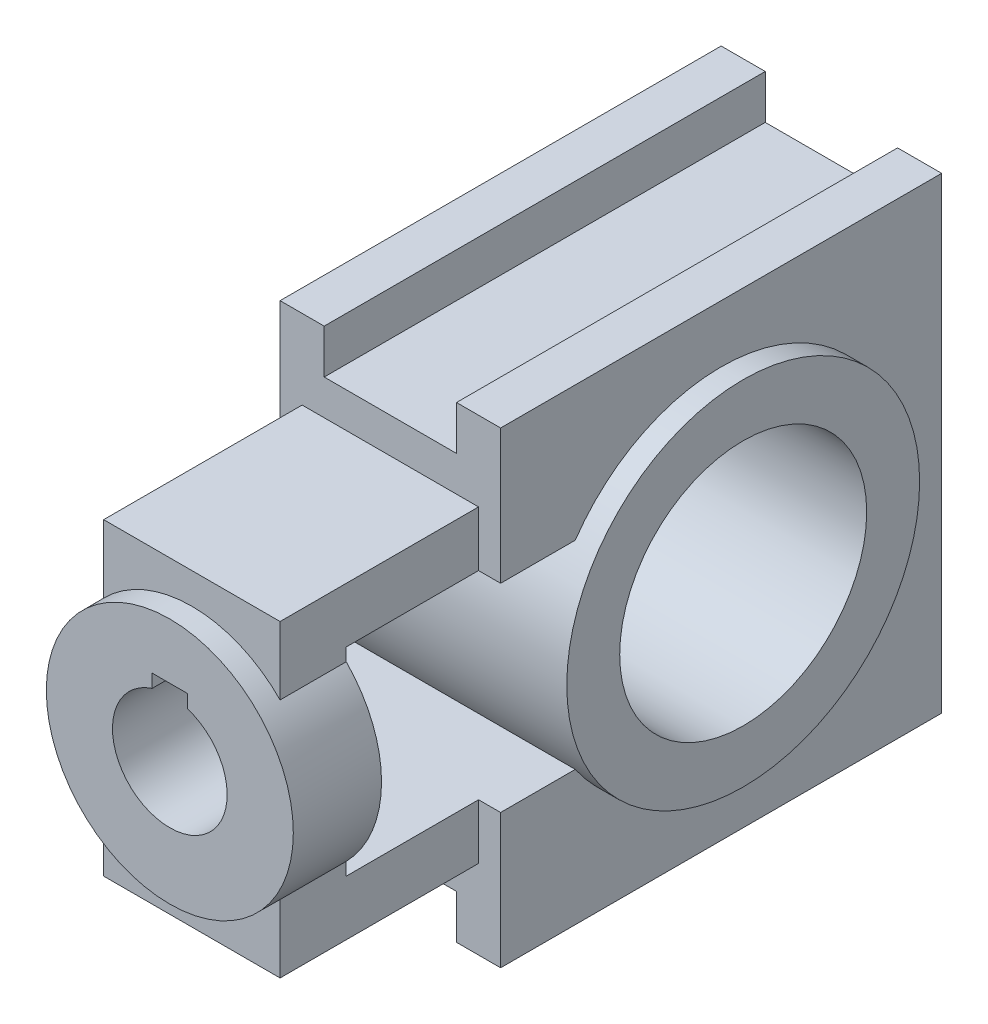
ISO-10303-21;
HEADER;
FILE_DESCRIPTION(('STEP AP214'),'2;1');
FILE_NAME('part.step','',(''),(''),'','','');
FILE_SCHEMA(('AUTOMOTIVE_DESIGN { 1 0 10303 214 1 1 1 1 }'));
ENDSEC;
DATA;
#1=APPLICATION_CONTEXT('core data for automotive mechanical design processes');
#2=APPLICATION_PROTOCOL_DEFINITION('international standard','automotive_design',2000,#1);
#3=PRODUCT_CONTEXT('',#1,'mechanical');
#4=PRODUCT('Part','Part','',(#3));
#5=PRODUCT_RELATED_PRODUCT_CATEGORY('part','',(#4));
#6=PRODUCT_DEFINITION_FORMATION('','',#4);
#7=PRODUCT_DEFINITION_CONTEXT('part definition',#1,'design');
#8=PRODUCT_DEFINITION('design','',#6,#7);
#9=PRODUCT_DEFINITION_SHAPE('','',#8);
#10=(LENGTH_UNIT() NAMED_UNIT(*) SI_UNIT(.MILLI.,.METRE.));
#11=(NAMED_UNIT(*) PLANE_ANGLE_UNIT() SI_UNIT($,.RADIAN.));
#12=(NAMED_UNIT(*) SI_UNIT($,.STERADIAN.) SOLID_ANGLE_UNIT());
#13=UNCERTAINTY_MEASURE_WITH_UNIT(LENGTH_MEASURE(1.E-05),#10,'distance_accuracy_value','');
#14=(GEOMETRIC_REPRESENTATION_CONTEXT(3) GLOBAL_UNCERTAINTY_ASSIGNED_CONTEXT((#13)) GLOBAL_UNIT_ASSIGNED_CONTEXT((#10,
#11,#12)) REPRESENTATION_CONTEXT('',''));
#15=CARTESIAN_POINT('',(0.,0.,0.));
#16=DIRECTION('',(0.,0.,1.));
#17=DIRECTION('',(1.,0.,0.));
#18=AXIS2_PLACEMENT_3D('',#15,#16,#17);
#19=CARTESIAN_POINT('',(25.,-53.,0.));
#20=DIRECTION('',(0.,1.,0.));
#21=DIRECTION('',(0.,0.,1.));
#22=AXIS2_PLACEMENT_3D('',#19,#20,#21);
#23=PLANE('',#22);
#24=DIRECTION('',(0.,0.,1.));
#25=VECTOR('',#24,1.);
#26=CARTESIAN_POINT('',(15.,-53.,-50.));
#27=LINE('',#26,#25);
#28=CARTESIAN_POINT('',(15.,-53.,-50.));
#29=VERTEX_POINT('',#28);
#30=CARTESIAN_POINT('',(15.,-53.,50.));
#31=VERTEX_POINT('',#30);
#32=EDGE_CURVE('E257',#29,#31,#27,.T.);
#33=ORIENTED_EDGE('',*,*,#32,.F.);
#34=DIRECTION('',(-1.,0.,0.));
#35=VECTOR('',#34,1.);
#36=CARTESIAN_POINT('',(25.,-53.,-50.));
#37=LINE('',#36,#35);
#38=CARTESIAN_POINT('',(25.,-53.,-50.));
#39=VERTEX_POINT('',#38);
#40=EDGE_CURVE('E280',#39,#29,#37,.T.);
#41=ORIENTED_EDGE('',*,*,#40,.F.);
#42=DIRECTION('',(0.,0.,-1.));
#43=VECTOR('',#42,1.);
#44=CARTESIAN_POINT('',(25.,-53.,0.));
#45=LINE('',#44,#43);
#46=CARTESIAN_POINT('',(25.,-53.,50.));
#47=VERTEX_POINT('',#46);
#48=EDGE_CURVE('E443',#47,#39,#45,.T.);
#49=ORIENTED_EDGE('',*,*,#48,.F.);
#50=DIRECTION('',(-1.,0.,0.));
#51=VECTOR('',#50,1.);
#52=CARTESIAN_POINT('',(25.,-53.,50.));
#53=LINE('',#52,#51);
#54=EDGE_CURVE('E289',#47,#31,#53,.T.);
#55=ORIENTED_EDGE('',*,*,#54,.T.);
#56=EDGE_LOOP('',(#33,#41,#49,#55));
#57=FACE_BOUND('',#56,.T.);
#58=ADVANCED_FACE('F41',(#57),#23,.F.);
#59=CARTESIAN_POINT('',(25.,53.,0.));
#60=DIRECTION('',(0.,1.,0.));
#61=DIRECTION('',(0.,0.,1.));
#62=AXIS2_PLACEMENT_3D('',#59,#60,#61);
#63=PLANE('',#62);
#64=DIRECTION('',(-1.,0.,0.));
#65=VECTOR('',#64,1.);
#66=CARTESIAN_POINT('',(25.,53.,-50.));
#67=LINE('',#66,#65);
#68=CARTESIAN_POINT('',(25.,53.,-50.));
#69=VERTEX_POINT('',#68);
#70=CARTESIAN_POINT('',(15.,53.,-50.));
#71=VERTEX_POINT('',#70);
#72=EDGE_CURVE('E279',#69,#71,#67,.T.);
#73=ORIENTED_EDGE('',*,*,#72,.T.);
#74=DIRECTION('',(0.,0.,1.));
#75=VECTOR('',#74,1.);
#76=CARTESIAN_POINT('',(15.,53.,-50.));
#77=LINE('',#76,#75);
#78=CARTESIAN_POINT('',(15.,53.,50.));
#79=VERTEX_POINT('',#78);
#80=EDGE_CURVE('E553',#71,#79,#77,.T.);
#81=ORIENTED_EDGE('',*,*,#80,.T.);
#82=DIRECTION('',(-1.,0.,0.));
#83=VECTOR('',#82,1.);
#84=CARTESIAN_POINT('',(25.,53.,50.));
#85=LINE('',#84,#83);
#86=CARTESIAN_POINT('',(25.,53.,50.));
#87=VERTEX_POINT('',#86);
#88=EDGE_CURVE('E483',#87,#79,#85,.T.);
#89=ORIENTED_EDGE('',*,*,#88,.F.);
#90=DIRECTION('',(0.,0.,-1.));
#91=VECTOR('',#90,1.);
#92=CARTESIAN_POINT('',(25.,53.,0.));
#93=LINE('',#92,#91);
#94=EDGE_CURVE('E450',#87,#69,#93,.T.);
#95=ORIENTED_EDGE('',*,*,#94,.T.);
#96=EDGE_LOOP('',(#73,#81,#89,#95));
#97=FACE_BOUND('',#96,.T.);
#98=ADVANCED_FACE('F578',(#97),#63,.T.);
#99=CARTESIAN_POINT('',(25.,0.,-50.));
#100=DIRECTION('',(0.,0.,-1.));
#101=DIRECTION('',(0.,1.,0.));
#102=AXIS2_PLACEMENT_3D('',#99,#100,#101);
#103=PLANE('',#102);
#104=DIRECTION('',(0.,1.,0.));
#105=VECTOR('',#104,1.);
#106=CARTESIAN_POINT('',(-15.,-53.,-50.));
#107=LINE('',#106,#105);
#108=CARTESIAN_POINT('',(-15.,-53.,-50.));
#109=VERTEX_POINT('',#108);
#110=CARTESIAN_POINT('',(-15.,-43.,-50.));
#111=VERTEX_POINT('',#110);
#112=EDGE_CURVE('E251',#109,#111,#107,.T.);
#113=ORIENTED_EDGE('',*,*,#112,.F.);
#114=CARTESIAN_POINT('',(-25.,-53.,-50.));
#115=VERTEX_POINT('',#114);
#116=EDGE_CURVE('E270',#109,#115,#37,.T.);
#117=ORIENTED_EDGE('',*,*,#116,.T.);
#118=DIRECTION('',(0.,-1.,0.));
#119=VECTOR('',#118,1.);
#120=CARTESIAN_POINT('',(-25.,0.,-50.));
#121=LINE('',#120,#119);
#122=CARTESIAN_POINT('',(-25.,53.,-50.));
#123=VERTEX_POINT('',#122);
#124=EDGE_CURVE('E470',#123,#115,#121,.T.);
#125=ORIENTED_EDGE('',*,*,#124,.F.);
#126=CARTESIAN_POINT('',(-15.,53.,-50.));
#127=VERTEX_POINT('',#126);
#128=EDGE_CURVE('E284',#127,#123,#67,.T.);
#129=ORIENTED_EDGE('',*,*,#128,.F.);
#130=DIRECTION('',(0.,-1.,0.));
#131=VECTOR('',#130,1.);
#132=CARTESIAN_POINT('',(-15.,53.,-50.));
#133=LINE('',#132,#131);
#134=CARTESIAN_POINT('',(-15.,43.,-50.));
#135=VERTEX_POINT('',#134);
#136=EDGE_CURVE('E585',#127,#135,#133,.T.);
#137=ORIENTED_EDGE('',*,*,#136,.T.);
#138=DIRECTION('',(1.,0.,0.));
#139=VECTOR('',#138,1.);
#140=CARTESIAN_POINT('',(-15.,43.,-50.));
#141=LINE('',#140,#139);
#142=CARTESIAN_POINT('',(15.,43.,-50.));
#143=VERTEX_POINT('',#142);
#144=EDGE_CURVE('E588',#135,#143,#141,.T.);
#145=ORIENTED_EDGE('',*,*,#144,.T.);
#146=DIRECTION('',(0.,1.,0.));
#147=VECTOR('',#146,1.);
#148=CARTESIAN_POINT('',(15.,53.,-50.));
#149=LINE('',#148,#147);
#150=EDGE_CURVE('E567',#143,#71,#149,.T.);
#151=ORIENTED_EDGE('',*,*,#150,.T.);
#152=ORIENTED_EDGE('',*,*,#72,.F.);
#153=DIRECTION('',(0.,-1.,0.));
#154=VECTOR('',#153,1.);
#155=CARTESIAN_POINT('',(25.,0.,-50.));
#156=LINE('',#155,#154);
#157=EDGE_CURVE('E447',#69,#39,#156,.T.);
#158=ORIENTED_EDGE('',*,*,#157,.T.);
#159=ORIENTED_EDGE('',*,*,#40,.T.);
#160=DIRECTION('',(0.,-1.,0.));
#161=VECTOR('',#160,1.);
#162=CARTESIAN_POINT('',(15.,-53.,-50.));
#163=LINE('',#162,#161);
#164=CARTESIAN_POINT('',(15.,-43.,-50.));
#165=VERTEX_POINT('',#164);
#166=EDGE_CURVE('E269',#165,#29,#163,.T.);
#167=ORIENTED_EDGE('',*,*,#166,.F.);
#168=DIRECTION('',(1.,0.,0.));
#169=VECTOR('',#168,1.);
#170=CARTESIAN_POINT('',(-15.,-43.,-50.));
#171=LINE('',#170,#169);
#172=EDGE_CURVE('E261',#111,#165,#171,.T.);
#173=ORIENTED_EDGE('',*,*,#172,.F.);
#174=EDGE_LOOP('',(#113,#117,#125,#129,#137,#145,#151,#152,#158,#159,#167,#173));
#175=FACE_BOUND('',#174,.T.);
#176=ADVANCED_FACE('F264',(#175),#103,.T.);
#177=CARTESIAN_POINT('',(25.,0.,50.));
#178=DIRECTION('',(0.,0.,-1.));
#179=DIRECTION('',(0.,1.,0.));
#180=AXIS2_PLACEMENT_3D('',#177,#178,#179);
#181=PLANE('',#180);
#182=DIRECTION('',(0.,-1.,0.));
#183=VECTOR('',#182,1.);
#184=CARTESIAN_POINT('',(-15.,53.,50.));
#185=LINE('',#184,#183);
#186=CARTESIAN_POINT('',(-15.,53.,50.));
#187=VERTEX_POINT('',#186);
#188=CARTESIAN_POINT('',(-15.,43.,50.));
#189=VERTEX_POINT('',#188);
#190=EDGE_CURVE('E63',#187,#189,#185,.T.);
#191=ORIENTED_EDGE('',*,*,#190,.F.);
#192=CARTESIAN_POINT('',(-25.,53.,50.));
#193=VERTEX_POINT('',#192);
#194=EDGE_CURVE('E485',#187,#193,#85,.T.);
#195=ORIENTED_EDGE('',*,*,#194,.T.);
#196=DIRECTION('',(0.,-1.,0.));
#197=VECTOR('',#196,1.);
#198=CARTESIAN_POINT('',(-25.,0.,50.));
#199=LINE('',#198,#197);
#200=CARTESIAN_POINT('',(-25.,22.5,50.));
#201=VERTEX_POINT('',#200);
#202=EDGE_CURVE('E471',#193,#201,#199,.T.);
#203=ORIENTED_EDGE('',*,*,#202,.T.);
#204=DIRECTION('',(-1.,0.,0.));
#205=VECTOR('',#204,1.);
#206=CARTESIAN_POINT('',(25.,22.5,50.));
#207=LINE('',#206,#205);
#208=CARTESIAN_POINT('',(-20.,22.5,50.));
#209=VERTEX_POINT('',#208);
#210=EDGE_CURVE('E479',#209,#201,#207,.T.);
#211=ORIENTED_EDGE('',*,*,#210,.F.);
#212=DIRECTION('',(0.,1.,0.));
#213=VECTOR('',#212,1.);
#214=CARTESIAN_POINT('',(-20.,22.5,50.));
#215=LINE('',#214,#213);
#216=CARTESIAN_POINT('',(-20.,35.,50.));
#217=VERTEX_POINT('',#216);
#218=EDGE_CURVE('E401',#209,#217,#215,.T.);
#219=ORIENTED_EDGE('',*,*,#218,.T.);
#220=DIRECTION('',(-1.,0.,0.));
#221=VECTOR('',#220,1.);
#222=CARTESIAN_POINT('',(20.,35.,50.));
#223=LINE('',#222,#221);
#224=CARTESIAN_POINT('',(20.,35.,50.));
#225=VERTEX_POINT('',#224);
#226=EDGE_CURVE('E433',#225,#217,#223,.T.);
#227=ORIENTED_EDGE('',*,*,#226,.F.);
#228=DIRECTION('',(0.,1.,0.));
#229=VECTOR('',#228,1.);
#230=CARTESIAN_POINT('',(20.,22.5,50.));
#231=LINE('',#230,#229);
#232=CARTESIAN_POINT('',(20.,22.5,50.));
#233=VERTEX_POINT('',#232);
#234=EDGE_CURVE('E404',#233,#225,#231,.T.);
#235=ORIENTED_EDGE('',*,*,#234,.F.);
#236=CARTESIAN_POINT('',(25.,22.5,50.));
#237=VERTEX_POINT('',#236);
#238=EDGE_CURVE('E477',#237,#233,#207,.T.);
#239=ORIENTED_EDGE('',*,*,#238,.F.);
#240=DIRECTION('',(0.,-1.,0.));
#241=VECTOR('',#240,1.);
#242=CARTESIAN_POINT('',(25.,0.,50.));
#243=LINE('',#242,#241);
#244=EDGE_CURVE('E455',#87,#237,#243,.T.);
#245=ORIENTED_EDGE('',*,*,#244,.F.);
#246=ORIENTED_EDGE('',*,*,#88,.T.);
#247=DIRECTION('',(0.,1.,0.));
#248=VECTOR('',#247,1.);
#249=CARTESIAN_POINT('',(15.,53.,50.));
#250=LINE('',#249,#248);
#251=CARTESIAN_POINT('',(15.,43.,50.));
#252=VERTEX_POINT('',#251);
#253=EDGE_CURVE('E562',#252,#79,#250,.T.);
#254=ORIENTED_EDGE('',*,*,#253,.F.);
#255=DIRECTION('',(1.,0.,0.));
#256=VECTOR('',#255,1.);
#257=CARTESIAN_POINT('',(-15.,43.,50.));
#258=LINE('',#257,#256);
#259=EDGE_CURVE('E584',#189,#252,#258,.T.);
#260=ORIENTED_EDGE('',*,*,#259,.F.);
#261=EDGE_LOOP('',(#191,#195,#203,#211,#219,#227,#235,#239,#245,#246,#254,#260));
#262=FACE_BOUND('',#261,.T.);
#263=ADVANCED_FACE('F489',(#262),#181,.F.);
#264=CARTESIAN_POINT('',(25.,0.,50.));
#265=DIRECTION('',(0.,0.,-1.));
#266=DIRECTION('',(0.,1.,0.));
#267=AXIS2_PLACEMENT_3D('',#264,#265,#266);
#268=PLANE('',#267);
#269=CARTESIAN_POINT('',(-15.,-53.,50.));
#270=VERTEX_POINT('',#269);
#271=CARTESIAN_POINT('',(-25.,-53.,50.));
#272=VERTEX_POINT('',#271);
#273=EDGE_CURVE('E281',#270,#272,#53,.T.);
#274=ORIENTED_EDGE('',*,*,#273,.F.);
#275=DIRECTION('',(0.,1.,0.));
#276=VECTOR('',#275,1.);
#277=CARTESIAN_POINT('',(-15.,-53.,50.));
#278=LINE('',#277,#276);
#279=CARTESIAN_POINT('',(-15.,-43.,50.));
#280=VERTEX_POINT('',#279);
#281=EDGE_CURVE('E258',#270,#280,#278,.T.);
#282=ORIENTED_EDGE('',*,*,#281,.T.);
#283=DIRECTION('',(1.,0.,0.));
#284=VECTOR('',#283,1.);
#285=CARTESIAN_POINT('',(-15.,-43.,50.));
#286=LINE('',#285,#284);
#287=CARTESIAN_POINT('',(15.,-43.,50.));
#288=VERTEX_POINT('',#287);
#289=EDGE_CURVE('E271',#280,#288,#286,.T.);
#290=ORIENTED_EDGE('',*,*,#289,.T.);
#291=DIRECTION('',(0.,-1.,0.));
#292=VECTOR('',#291,1.);
#293=CARTESIAN_POINT('',(15.,-53.,50.));
#294=LINE('',#293,#292);
#295=EDGE_CURVE('E57',#288,#31,#294,.T.);
#296=ORIENTED_EDGE('',*,*,#295,.T.);
#297=ORIENTED_EDGE('',*,*,#54,.F.);
#298=DIRECTION('',(0.,-1.,0.));
#299=VECTOR('',#298,1.);
#300=CARTESIAN_POINT('',(25.,0.,50.));
#301=LINE('',#300,#299);
#302=CARTESIAN_POINT('',(25.,-22.5,50.));
#303=VERTEX_POINT('',#302);
#304=EDGE_CURVE('E444',#303,#47,#301,.T.);
#305=ORIENTED_EDGE('',*,*,#304,.F.);
#306=DIRECTION('',(-1.,0.,0.));
#307=VECTOR('',#306,1.);
#308=CARTESIAN_POINT('',(25.,-22.5,50.));
#309=LINE('',#308,#307);
#310=CARTESIAN_POINT('',(20.,-22.5,50.));
#311=VERTEX_POINT('',#310);
#312=EDGE_CURVE('E292',#303,#311,#309,.T.);
#313=ORIENTED_EDGE('',*,*,#312,.T.);
#314=DIRECTION('',(0.,-1.,0.));
#315=VECTOR('',#314,1.);
#316=CARTESIAN_POINT('',(20.,-22.5,50.));
#317=LINE('',#316,#315);
#318=CARTESIAN_POINT('',(20.,-35.,50.));
#319=VERTEX_POINT('',#318);
#320=EDGE_CURVE('E354',#311,#319,#317,.T.);
#321=ORIENTED_EDGE('',*,*,#320,.T.);
#322=DIRECTION('',(-1.,0.,0.));
#323=VECTOR('',#322,1.);
#324=CARTESIAN_POINT('',(20.,-35.,50.));
#325=LINE('',#324,#323);
#326=CARTESIAN_POINT('',(-20.,-35.,50.));
#327=VERTEX_POINT('',#326);
#328=EDGE_CURVE('E353',#319,#327,#325,.T.);
#329=ORIENTED_EDGE('',*,*,#328,.T.);
#330=DIRECTION('',(0.,-1.,0.));
#331=VECTOR('',#330,1.);
#332=CARTESIAN_POINT('',(-20.,-22.5,50.));
#333=LINE('',#332,#331);
#334=CARTESIAN_POINT('',(-20.,-22.5,50.));
#335=VERTEX_POINT('',#334);
#336=EDGE_CURVE('E346',#335,#327,#333,.T.);
#337=ORIENTED_EDGE('',*,*,#336,.F.);
#338=CARTESIAN_POINT('',(-25.,-22.5,50.));
#339=VERTEX_POINT('',#338);
#340=EDGE_CURVE('E288',#335,#339,#309,.T.);
#341=ORIENTED_EDGE('',*,*,#340,.T.);
#342=DIRECTION('',(0.,-1.,0.));
#343=VECTOR('',#342,1.);
#344=CARTESIAN_POINT('',(-25.,0.,50.));
#345=LINE('',#344,#343);
#346=EDGE_CURVE('E463',#339,#272,#345,.T.);
#347=ORIENTED_EDGE('',*,*,#346,.T.);
#348=EDGE_LOOP('',(#274,#282,#290,#296,#297,#305,#313,#321,#329,#337,#341,#347));
#349=FACE_BOUND('',#348,.T.);
#350=ADVANCED_FACE('F566',(#349),#268,.F.);
#351=CARTESIAN_POINT('',(30.,0.,0.));
#352=DIRECTION('',(1.,0.,0.));
#353=DIRECTION('',(0.,0.,-1.));
#354=AXIS2_PLACEMENT_3D('',#351,#352,#353);
#355=PLANE('',#354);
#356=CARTESIAN_POINT('',(30.,0.,0.));
#357=DIRECTION('',(1.,0.,0.));
#358=DIRECTION('',(0.,0.,-1.));
#359=AXIS2_PLACEMENT_3D('',#356,#357,#358);
#360=CIRCLE('',#359,40.);
#361=CARTESIAN_POINT('',(30.,0.,-40.));
#362=VERTEX_POINT('',#361);
#363=EDGE_CURVE('E301',#362,#362,#360,.T.);
#364=ORIENTED_EDGE('',*,*,#363,.T.);
#365=EDGE_LOOP('',(#364));
#366=FACE_BOUND('',#365,.T.);
#367=CARTESIAN_POINT('',(30.,0.,0.));
#368=DIRECTION('',(1.,0.,0.));
#369=DIRECTION('',(0.,0.,-1.));
#370=AXIS2_PLACEMENT_3D('',#367,#368,#369);
#371=CIRCLE('',#370,28.);
#372=CARTESIAN_POINT('',(30.,0.,-28.));
#373=VERTEX_POINT('',#372);
#374=EDGE_CURVE('E299',#373,#373,#371,.T.);
#375=ORIENTED_EDGE('',*,*,#374,.F.);
#376=EDGE_LOOP('',(#375));
#377=FACE_BOUND('',#376,.T.);
#378=ADVANCED_FACE('F643',(#366,#377),#355,.T.);
#379=CARTESIAN_POINT('',(-30.,0.,0.));
#380=DIRECTION('',(1.,0.,0.));
#381=DIRECTION('',(0.,0.,-1.));
#382=AXIS2_PLACEMENT_3D('',#379,#380,#381);
#383=PLANE('',#382);
#384=CARTESIAN_POINT('',(-30.,0.,0.));
#385=DIRECTION('',(1.,0.,0.));
#386=DIRECTION('',(0.,0.,-1.));
#387=AXIS2_PLACEMENT_3D('',#384,#385,#386);
#388=CIRCLE('',#387,40.);
#389=CARTESIAN_POINT('',(-30.,0.,-40.));
#390=VERTEX_POINT('',#389);
#391=EDGE_CURVE('E302',#390,#390,#388,.T.);
#392=ORIENTED_EDGE('',*,*,#391,.F.);
#393=EDGE_LOOP('',(#392));
#394=FACE_BOUND('',#393,.T.);
#395=CARTESIAN_POINT('',(-30.,0.,0.));
#396=DIRECTION('',(1.,0.,0.));
#397=DIRECTION('',(0.,0.,-1.));
#398=AXIS2_PLACEMENT_3D('',#395,#396,#397);
#399=CIRCLE('',#398,28.);
#400=CARTESIAN_POINT('',(-30.,0.,-28.));
#401=VERTEX_POINT('',#400);
#402=EDGE_CURVE('E297',#401,#401,#399,.T.);
#403=ORIENTED_EDGE('',*,*,#402,.T.);
#404=EDGE_LOOP('',(#403));
#405=FACE_BOUND('',#404,.T.);
#406=ADVANCED_FACE('F641',(#394,#405),#383,.F.);
#407=CARTESIAN_POINT('',(30.,0.,0.));
#408=DIRECTION('',(-1.,0.,0.));
#409=DIRECTION('',(0.,0.,1.));
#410=AXIS2_PLACEMENT_3D('',#407,#408,#409);
#411=CYLINDRICAL_SURFACE('',#410,40.);
#412=DIRECTION('',(-1.,0.,0.));
#413=VECTOR('',#412,1.);
#414=CARTESIAN_POINT('',(25.,-22.5,33.0718913883074));
#415=LINE('',#414,#413);
#416=CARTESIAN_POINT('',(25.,-22.5,33.0718913883074));
#417=VERTEX_POINT('',#416);
#418=CARTESIAN_POINT('',(-25.,-22.5,33.0718913883074));
#419=VERTEX_POINT('',#418);
#420=EDGE_CURVE('E294',#417,#419,#415,.T.);
#421=ORIENTED_EDGE('',*,*,#420,.F.);
#422=CARTESIAN_POINT('',(25.,0.,0.));
#423=DIRECTION('',(1.,0.,0.));
#424=DIRECTION('',(0.,0.,-1.));
#425=AXIS2_PLACEMENT_3D('',#422,#423,#424);
#426=CIRCLE('',#425,40.);
#427=CARTESIAN_POINT('',(25.,22.5,33.0718913883074));
#428=VERTEX_POINT('',#427);
#429=EDGE_CURVE('E440',#417,#428,#426,.T.);
#430=ORIENTED_EDGE('',*,*,#429,.T.);
#431=DIRECTION('',(-1.,0.,0.));
#432=VECTOR('',#431,1.);
#433=CARTESIAN_POINT('',(25.,22.5,33.0718913883074));
#434=LINE('',#433,#432);
#435=CARTESIAN_POINT('',(-25.,22.5,33.0718913883074));
#436=VERTEX_POINT('',#435);
#437=EDGE_CURVE('E456',#428,#436,#434,.T.);
#438=ORIENTED_EDGE('',*,*,#437,.T.);
#439=CARTESIAN_POINT('',(-25.,0.,0.));
#440=DIRECTION('',(1.,0.,0.));
#441=DIRECTION('',(0.,0.,-1.));
#442=AXIS2_PLACEMENT_3D('',#439,#440,#441);
#443=CIRCLE('',#442,40.);
#444=EDGE_CURVE('E436',#419,#436,#443,.T.);
#445=ORIENTED_EDGE('',*,*,#444,.F.);
#446=EDGE_LOOP('',(#421,#430,#438,#445));
#447=FACE_BOUND('',#446,.T.);
#448=ORIENTED_EDGE('',*,*,#363,.F.);
#449=EDGE_LOOP('',(#448));
#450=FACE_BOUND('',#449,.T.);
#451=ORIENTED_EDGE('',*,*,#391,.T.);
#452=EDGE_LOOP('',(#451));
#453=FACE_BOUND('',#452,.T.);
#454=ADVANCED_FACE('F43',(#447,#450,#453),#411,.T.);
#455=CARTESIAN_POINT('',(30.,0.,0.));
#456=DIRECTION('',(-1.,0.,0.));
#457=DIRECTION('',(0.,0.,1.));
#458=AXIS2_PLACEMENT_3D('',#455,#456,#457);
#459=CYLINDRICAL_SURFACE('',#458,28.);
#460=ORIENTED_EDGE('',*,*,#374,.T.);
#461=EDGE_LOOP('',(#460));
#462=FACE_BOUND('',#461,.T.);
#463=ORIENTED_EDGE('',*,*,#402,.F.);
#464=EDGE_LOOP('',(#463));
#465=FACE_BOUND('',#464,.T.);
#466=ADVANCED_FACE('F632',(#462,#465),#459,.F.);
#467=CARTESIAN_POINT('',(25.,-22.5,0.));
#468=DIRECTION('',(0.,1.,0.));
#469=DIRECTION('',(0.,0.,1.));
#470=AXIS2_PLACEMENT_3D('',#467,#468,#469);
#471=PLANE('',#470);
#472=DIRECTION('',(0.,0.,-1.));
#473=VECTOR('',#472,1.);
#474=CARTESIAN_POINT('',(-25.,-22.5,0.));
#475=LINE('',#474,#473);
#476=EDGE_CURVE('E461',#339,#419,#475,.T.);
#477=ORIENTED_EDGE('',*,*,#476,.F.);
#478=ORIENTED_EDGE('',*,*,#340,.F.);
#479=DIRECTION('',(0.,0.,-1.));
#480=VECTOR('',#479,1.);
#481=CARTESIAN_POINT('',(-20.,-22.5,80.));
#482=LINE('',#481,#480);
#483=CARTESIAN_POINT('',(-20.,-22.5,80.));
#484=VERTEX_POINT('',#483);
#485=EDGE_CURVE('E341',#484,#335,#482,.T.);
#486=ORIENTED_EDGE('',*,*,#485,.F.);
#487=DIRECTION('',(-1.,0.,0.));
#488=VECTOR('',#487,1.);
#489=CARTESIAN_POINT('',(20.,-22.5,80.));
#490=LINE('',#489,#488);
#491=CARTESIAN_POINT('',(20.,-22.5,80.));
#492=VERTEX_POINT('',#491);
#493=EDGE_CURVE('E345',#492,#484,#490,.T.);
#494=ORIENTED_EDGE('',*,*,#493,.F.);
#495=DIRECTION('',(0.,0.,-1.));
#496=VECTOR('',#495,1.);
#497=CARTESIAN_POINT('',(20.,-22.5,80.));
#498=LINE('',#497,#496);
#499=EDGE_CURVE('E550',#492,#311,#498,.T.);
#500=ORIENTED_EDGE('',*,*,#499,.T.);
#501=ORIENTED_EDGE('',*,*,#312,.F.);
#502=DIRECTION('',(0.,0.,-1.));
#503=VECTOR('',#502,1.);
#504=CARTESIAN_POINT('',(25.,-22.5,0.));
#505=LINE('',#504,#503);
#506=EDGE_CURVE('E438',#303,#417,#505,.T.);
#507=ORIENTED_EDGE('',*,*,#506,.T.);
#508=ORIENTED_EDGE('',*,*,#420,.T.);
#509=EDGE_LOOP('',(#477,#478,#486,#494,#500,#501,#507,#508));
#510=FACE_BOUND('',#509,.T.);
#511=ADVANCED_FACE('F509',(#510),#471,.T.);
#512=ORIENTED_EDGE('',*,*,#116,.F.);
#513=DIRECTION('',(0.,0.,1.));
#514=VECTOR('',#513,1.);
#515=CARTESIAN_POINT('',(-15.,-53.,-50.));
#516=LINE('',#515,#514);
#517=EDGE_CURVE('E246',#109,#270,#516,.T.);
#518=ORIENTED_EDGE('',*,*,#517,.T.);
#519=ORIENTED_EDGE('',*,*,#273,.T.);
#520=DIRECTION('',(0.,0.,-1.));
#521=VECTOR('',#520,1.);
#522=CARTESIAN_POINT('',(-25.,-53.,0.));
#523=LINE('',#522,#521);
#524=EDGE_CURVE('E274',#272,#115,#523,.T.);
#525=ORIENTED_EDGE('',*,*,#524,.T.);
#526=EDGE_LOOP('',(#512,#518,#519,#525));
#527=FACE_BOUND('',#526,.T.);
#528=ADVANCED_FACE('F272',(#527),#23,.F.);
#529=DIRECTION('',(0.,0.,1.));
#530=VECTOR('',#529,1.);
#531=CARTESIAN_POINT('',(-15.,53.,-50.));
#532=LINE('',#531,#530);
#533=EDGE_CURVE('E498',#127,#187,#532,.T.);
#534=ORIENTED_EDGE('',*,*,#533,.F.);
#535=ORIENTED_EDGE('',*,*,#128,.T.);
#536=DIRECTION('',(0.,0.,-1.));
#537=VECTOR('',#536,1.);
#538=CARTESIAN_POINT('',(-25.,53.,0.));
#539=LINE('',#538,#537);
#540=EDGE_CURVE('E468',#193,#123,#539,.T.);
#541=ORIENTED_EDGE('',*,*,#540,.F.);
#542=ORIENTED_EDGE('',*,*,#194,.F.);
#543=EDGE_LOOP('',(#534,#535,#541,#542));
#544=FACE_BOUND('',#543,.T.);
#545=ADVANCED_FACE('F499',(#544),#63,.T.);
#546=CARTESIAN_POINT('',(25.,22.5,0.));
#547=DIRECTION('',(0.,1.,0.));
#548=DIRECTION('',(0.,0.,1.));
#549=AXIS2_PLACEMENT_3D('',#546,#547,#548);
#550=PLANE('',#549);
#551=DIRECTION('',(0.,0.,-1.));
#552=VECTOR('',#551,1.);
#553=CARTESIAN_POINT('',(-25.,22.5,0.));
#554=LINE('',#553,#552);
#555=EDGE_CURVE('E439',#201,#436,#554,.T.);
#556=ORIENTED_EDGE('',*,*,#555,.T.);
#557=ORIENTED_EDGE('',*,*,#437,.F.);
#558=DIRECTION('',(0.,0.,-1.));
#559=VECTOR('',#558,1.);
#560=CARTESIAN_POINT('',(25.,22.5,0.));
#561=LINE('',#560,#559);
#562=EDGE_CURVE('E453',#237,#428,#561,.T.);
#563=ORIENTED_EDGE('',*,*,#562,.F.);
#564=ORIENTED_EDGE('',*,*,#238,.T.);
#565=DIRECTION('',(0.,0.,-1.));
#566=VECTOR('',#565,1.);
#567=CARTESIAN_POINT('',(20.,22.5,80.));
#568=LINE('',#567,#566);
#569=CARTESIAN_POINT('',(20.,22.5,80.));
#570=VERTEX_POINT('',#569);
#571=EDGE_CURVE('E413',#570,#233,#568,.T.);
#572=ORIENTED_EDGE('',*,*,#571,.F.);
#573=DIRECTION('',(-1.,0.,0.));
#574=VECTOR('',#573,1.);
#575=CARTESIAN_POINT('',(20.,22.5,80.));
#576=LINE('',#575,#574);
#577=CARTESIAN_POINT('',(-20.,22.5,80.));
#578=VERTEX_POINT('',#577);
#579=EDGE_CURVE('E416',#570,#578,#576,.T.);
#580=ORIENTED_EDGE('',*,*,#579,.T.);
#581=DIRECTION('',(0.,0.,-1.));
#582=VECTOR('',#581,1.);
#583=CARTESIAN_POINT('',(-20.,22.5,80.));
#584=LINE('',#583,#582);
#585=EDGE_CURVE('E409',#578,#209,#584,.T.);
#586=ORIENTED_EDGE('',*,*,#585,.T.);
#587=ORIENTED_EDGE('',*,*,#210,.T.);
#588=EDGE_LOOP('',(#556,#557,#563,#564,#572,#580,#586,#587));
#589=FACE_BOUND('',#588,.T.);
#590=ADVANCED_FACE('F518',(#589),#550,.F.);
#591=CARTESIAN_POINT('',(25.,0.,0.));
#592=DIRECTION('',(1.,0.,0.));
#593=DIRECTION('',(0.,0.,-1.));
#594=AXIS2_PLACEMENT_3D('',#591,#592,#593);
#595=PLANE('',#594);
#596=ORIENTED_EDGE('',*,*,#429,.F.);
#597=ORIENTED_EDGE('',*,*,#506,.F.);
#598=ORIENTED_EDGE('',*,*,#304,.T.);
#599=ORIENTED_EDGE('',*,*,#48,.T.);
#600=ORIENTED_EDGE('',*,*,#157,.F.);
#601=ORIENTED_EDGE('',*,*,#94,.F.);
#602=ORIENTED_EDGE('',*,*,#244,.T.);
#603=ORIENTED_EDGE('',*,*,#562,.T.);
#604=EDGE_LOOP('',(#596,#597,#598,#599,#600,#601,#602,#603));
#605=FACE_BOUND('',#604,.T.);
#606=ADVANCED_FACE('F511',(#605),#595,.T.);
#607=CARTESIAN_POINT('',(-25.,0.,0.));
#608=DIRECTION('',(1.,0.,0.));
#609=DIRECTION('',(0.,0.,-1.));
#610=AXIS2_PLACEMENT_3D('',#607,#608,#609);
#611=PLANE('',#610);
#612=ORIENTED_EDGE('',*,*,#444,.T.);
#613=ORIENTED_EDGE('',*,*,#555,.F.);
#614=ORIENTED_EDGE('',*,*,#202,.F.);
#615=ORIENTED_EDGE('',*,*,#540,.T.);
#616=ORIENTED_EDGE('',*,*,#124,.T.);
#617=ORIENTED_EDGE('',*,*,#524,.F.);
#618=ORIENTED_EDGE('',*,*,#346,.F.);
#619=ORIENTED_EDGE('',*,*,#476,.T.);
#620=EDGE_LOOP('',(#612,#613,#614,#615,#616,#617,#618,#619));
#621=FACE_BOUND('',#620,.T.);
#622=ADVANCED_FACE('F500',(#621),#611,.F.);
#623=CARTESIAN_POINT('',(20.,35.,50.));
#624=DIRECTION('',(0.,-1.,0.));
#625=DIRECTION('',(0.,0.,-1.));
#626=AXIS2_PLACEMENT_3D('',#623,#624,#625);
#627=PLANE('',#626);
#628=DIRECTION('',(0.,0.,1.));
#629=VECTOR('',#628,1.);
#630=CARTESIAN_POINT('',(-20.,35.,50.));
#631=LINE('',#630,#629);
#632=CARTESIAN_POINT('',(-20.,35.,95.));
#633=VERTEX_POINT('',#632);
#634=EDGE_CURVE('E419',#217,#633,#631,.T.);
#635=ORIENTED_EDGE('',*,*,#634,.T.);
#636=DIRECTION('',(-1.,0.,0.));
#637=VECTOR('',#636,1.);
#638=CARTESIAN_POINT('',(20.,35.,95.));
#639=LINE('',#638,#637);
#640=CARTESIAN_POINT('',(20.,35.,95.));
#641=VERTEX_POINT('',#640);
#642=EDGE_CURVE('E429',#641,#633,#639,.T.);
#643=ORIENTED_EDGE('',*,*,#642,.F.);
#644=DIRECTION('',(0.,0.,1.));
#645=VECTOR('',#644,1.);
#646=CARTESIAN_POINT('',(20.,35.,50.));
#647=LINE('',#646,#645);
#648=EDGE_CURVE('E407',#225,#641,#647,.T.);
#649=ORIENTED_EDGE('',*,*,#648,.F.);
#650=ORIENTED_EDGE('',*,*,#226,.T.);
#651=EDGE_LOOP('',(#635,#643,#649,#650));
#652=FACE_BOUND('',#651,.T.);
#653=ADVANCED_FACE('F529',(#652),#627,.F.);
#654=CARTESIAN_POINT('',(20.,35.,95.));
#655=DIRECTION('',(0.,0.,-1.));
#656=DIRECTION('',(-1.,0.,0.));
#657=AXIS2_PLACEMENT_3D('',#654,#655,#656);
#658=PLANE('',#657);
#659=DIRECTION('',(0.,-1.,0.));
#660=VECTOR('',#659,1.);
#661=CARTESIAN_POINT('',(-20.,35.,95.));
#662=LINE('',#661,#660);
#663=CARTESIAN_POINT('',(-20.,19.5959179422654,95.));
#664=VERTEX_POINT('',#663);
#665=EDGE_CURVE('E425',#633,#664,#662,.T.);
#666=ORIENTED_EDGE('',*,*,#665,.T.);
#667=CARTESIAN_POINT('',(0.,0.,95.));
#668=DIRECTION('',(0.,0.,-1.));
#669=DIRECTION('',(-1.,0.,0.));
#670=AXIS2_PLACEMENT_3D('',#667,#668,#669);
#671=CIRCLE('',#670,28.);
#672=CARTESIAN_POINT('',(20.,19.5959179422654,95.));
#673=VERTEX_POINT('',#672);
#674=EDGE_CURVE('E395',#664,#673,#671,.T.);
#675=ORIENTED_EDGE('',*,*,#674,.T.);
#676=DIRECTION('',(0.,-1.,0.));
#677=VECTOR('',#676,1.);
#678=CARTESIAN_POINT('',(20.,35.,95.));
#679=LINE('',#678,#677);
#680=EDGE_CURVE('E410',#641,#673,#679,.T.);
#681=ORIENTED_EDGE('',*,*,#680,.F.);
#682=ORIENTED_EDGE('',*,*,#642,.T.);
#683=EDGE_LOOP('',(#666,#675,#681,#682));
#684=FACE_BOUND('',#683,.T.);
#685=ADVANCED_FACE('F537',(#684),#658,.F.);
#686=CARTESIAN_POINT('',(20.,17.,80.));
#687=DIRECTION('',(0.,0.,1.));
#688=DIRECTION('',(1.,0.,0.));
#689=AXIS2_PLACEMENT_3D('',#686,#687,#688);
#690=PLANE('',#689);
#691=CARTESIAN_POINT('',(0.,0.,80.));
#692=DIRECTION('',(0.,0.,1.));
#693=DIRECTION('',(1.,0.,0.));
#694=AXIS2_PLACEMENT_3D('',#691,#692,#693);
#695=CIRCLE('',#694,28.);
#696=CARTESIAN_POINT('',(20.,-19.5959179422654,80.));
#697=VERTEX_POINT('',#696);
#698=CARTESIAN_POINT('',(20.,19.5959179422654,80.));
#699=VERTEX_POINT('',#698);
#700=EDGE_CURVE('E397',#697,#699,#695,.T.);
#701=ORIENTED_EDGE('',*,*,#700,.F.);
#702=DIRECTION('',(0.,-1.,0.));
#703=VECTOR('',#702,1.);
#704=CARTESIAN_POINT('',(20.,-17.,80.));
#705=LINE('',#704,#703);
#706=EDGE_CURVE('E539',#697,#492,#705,.T.);
#707=ORIENTED_EDGE('',*,*,#706,.T.);
#708=ORIENTED_EDGE('',*,*,#493,.T.);
#709=DIRECTION('',(0.,-1.,0.));
#710=VECTOR('',#709,1.);
#711=CARTESIAN_POINT('',(-20.,-17.,80.));
#712=LINE('',#711,#710);
#713=CARTESIAN_POINT('',(-20.,-19.5959179422654,80.));
#714=VERTEX_POINT('',#713);
#715=EDGE_CURVE('E333',#714,#484,#712,.T.);
#716=ORIENTED_EDGE('',*,*,#715,.F.);
#717=CARTESIAN_POINT('',(-20.,19.5959179422654,80.));
#718=VERTEX_POINT('',#717);
#719=EDGE_CURVE('E329',#718,#714,#695,.T.);
#720=ORIENTED_EDGE('',*,*,#719,.F.);
#721=DIRECTION('',(0.,1.,0.));
#722=VECTOR('',#721,1.);
#723=CARTESIAN_POINT('',(-20.,17.,80.));
#724=LINE('',#723,#722);
#725=EDGE_CURVE('E422',#718,#578,#724,.T.);
#726=ORIENTED_EDGE('',*,*,#725,.T.);
#727=ORIENTED_EDGE('',*,*,#579,.F.);
#728=DIRECTION('',(0.,1.,0.));
#729=VECTOR('',#728,1.);
#730=CARTESIAN_POINT('',(20.,17.,80.));
#731=LINE('',#730,#729);
#732=EDGE_CURVE('E415',#699,#570,#731,.T.);
#733=ORIENTED_EDGE('',*,*,#732,.F.);
#734=EDGE_LOOP('',(#701,#707,#708,#716,#720,#726,#727,#733));
#735=FACE_BOUND('',#734,.T.);
#736=DIRECTION('',(0.,-1.,0.));
#737=VECTOR('',#736,1.);
#738=CARTESIAN_POINT('',(-4.,12.369316876853,80.));
#739=LINE('',#738,#737);
#740=CARTESIAN_POINT('',(-4.,15.369316876853,80.));
#741=VERTEX_POINT('',#740);
#742=CARTESIAN_POINT('',(-4.,12.369316876853,80.));
#743=VERTEX_POINT('',#742);
#744=EDGE_CURVE('E375',#741,#743,#739,.T.);
#745=ORIENTED_EDGE('',*,*,#744,.T.);
#746=CARTESIAN_POINT('',(0.,0.,80.));
#747=DIRECTION('',(0.,0.,1.));
#748=DIRECTION('',(1.,0.,0.));
#749=AXIS2_PLACEMENT_3D('',#746,#747,#748);
#750=CIRCLE('',#749,13.);
#751=CARTESIAN_POINT('',(4.,12.369316876853,80.));
#752=VERTEX_POINT('',#751);
#753=EDGE_CURVE('E362',#743,#752,#750,.T.);
#754=ORIENTED_EDGE('',*,*,#753,.T.);
#755=DIRECTION('',(0.,1.,0.));
#756=VECTOR('',#755,1.);
#757=CARTESIAN_POINT('',(4.,12.369316876853,80.));
#758=LINE('',#757,#756);
#759=CARTESIAN_POINT('',(4.,15.369316876853,80.));
#760=VERTEX_POINT('',#759);
#761=EDGE_CURVE('E364',#752,#760,#758,.T.);
#762=ORIENTED_EDGE('',*,*,#761,.T.);
#763=DIRECTION('',(-1.,0.,0.));
#764=VECTOR('',#763,1.);
#765=CARTESIAN_POINT('',(-4.,15.369316876853,80.));
#766=LINE('',#765,#764);
#767=EDGE_CURVE('E369',#760,#741,#766,.T.);
#768=ORIENTED_EDGE('',*,*,#767,.T.);
#769=EDGE_LOOP('',(#745,#754,#762,#768));
#770=FACE_BOUND('',#769,.T.);
#771=ADVANCED_FACE('F338',(#735,#770),#690,.F.);
#772=CARTESIAN_POINT('',(20.,0.,0.));
#773=DIRECTION('',(1.,0.,0.));
#774=DIRECTION('',(0.,0.,-1.));
#775=AXIS2_PLACEMENT_3D('',#772,#773,#774);
#776=PLANE('',#775);
#777=DIRECTION('',(0.,0.,1.));
#778=VECTOR('',#777,1.);
#779=CARTESIAN_POINT('',(20.,19.5959179422654,80.));
#780=LINE('',#779,#778);
#781=EDGE_CURVE('E402',#699,#673,#780,.T.);
#782=ORIENTED_EDGE('',*,*,#781,.F.);
#783=ORIENTED_EDGE('',*,*,#732,.T.);
#784=ORIENTED_EDGE('',*,*,#571,.T.);
#785=ORIENTED_EDGE('',*,*,#234,.T.);
#786=ORIENTED_EDGE('',*,*,#648,.T.);
#787=ORIENTED_EDGE('',*,*,#680,.T.);
#788=EDGE_LOOP('',(#782,#783,#784,#785,#786,#787));
#789=FACE_BOUND('',#788,.T.);
#790=ADVANCED_FACE('F534',(#789),#776,.T.);
#791=CARTESIAN_POINT('',(-20.,0.,0.));
#792=DIRECTION('',(1.,0.,0.));
#793=DIRECTION('',(0.,0.,-1.));
#794=AXIS2_PLACEMENT_3D('',#791,#792,#793);
#795=PLANE('',#794);
#796=ORIENTED_EDGE('',*,*,#725,.F.);
#797=DIRECTION('',(0.,0.,1.));
#798=VECTOR('',#797,1.);
#799=CARTESIAN_POINT('',(-20.,19.5959179422654,80.));
#800=LINE('',#799,#798);
#801=EDGE_CURVE('E307',#718,#664,#800,.T.);
#802=ORIENTED_EDGE('',*,*,#801,.T.);
#803=ORIENTED_EDGE('',*,*,#665,.F.);
#804=ORIENTED_EDGE('',*,*,#634,.F.);
#805=ORIENTED_EDGE('',*,*,#218,.F.);
#806=ORIENTED_EDGE('',*,*,#585,.F.);
#807=EDGE_LOOP('',(#796,#802,#803,#804,#805,#806));
#808=FACE_BOUND('',#807,.T.);
#809=ADVANCED_FACE('F527',(#808),#795,.F.);
#810=CARTESIAN_POINT('',(0.,0.,80.));
#811=DIRECTION('',(0.,0.,1.));
#812=DIRECTION('',(1.,0.,0.));
#813=AXIS2_PLACEMENT_3D('',#810,#811,#812);
#814=CYLINDRICAL_SURFACE('',#813,28.);
#815=DIRECTION('',(0.,0.,1.));
#816=VECTOR('',#815,1.);
#817=CARTESIAN_POINT('',(20.,-19.5959179422654,80.));
#818=LINE('',#817,#816);
#819=CARTESIAN_POINT('',(20.,-19.5959179422654,95.));
#820=VERTEX_POINT('',#819);
#821=EDGE_CURVE('E11',#697,#820,#818,.T.);
#822=ORIENTED_EDGE('',*,*,#821,.F.);
#823=ORIENTED_EDGE('',*,*,#700,.T.);
#824=ORIENTED_EDGE('',*,*,#781,.T.);
#825=ORIENTED_EDGE('',*,*,#674,.F.);
#826=ORIENTED_EDGE('',*,*,#801,.F.);
#827=ORIENTED_EDGE('',*,*,#719,.T.);
#828=DIRECTION('',(0.,0.,1.));
#829=VECTOR('',#828,1.);
#830=CARTESIAN_POINT('',(-20.,-19.5959179422654,80.));
#831=LINE('',#830,#829);
#832=CARTESIAN_POINT('',(-20.,-19.5959179422654,95.));
#833=VERTEX_POINT('',#832);
#834=EDGE_CURVE('E315',#714,#833,#831,.T.);
#835=ORIENTED_EDGE('',*,*,#834,.T.);
#836=CARTESIAN_POINT('',(0.,0.,95.));
#837=DIRECTION('',(0.,0.,1.));
#838=DIRECTION('',(1.,0.,0.));
#839=AXIS2_PLACEMENT_3D('',#836,#837,#838);
#840=CIRCLE('',#839,28.);
#841=EDGE_CURVE('E47',#820,#833,#840,.F.);
#842=ORIENTED_EDGE('',*,*,#841,.F.);
#843=EDGE_LOOP('',(#822,#823,#824,#825,#826,#827,#835,#842));
#844=FACE_BOUND('',#843,.T.);
#845=CARTESIAN_POINT('',(0.,0.,100.));
#846=DIRECTION('',(0.,0.,1.));
#847=DIRECTION('',(1.,0.,0.));
#848=AXIS2_PLACEMENT_3D('',#845,#846,#847);
#849=CIRCLE('',#848,28.);
#850=CARTESIAN_POINT('',(28.,0.,100.));
#851=VERTEX_POINT('',#850);
#852=EDGE_CURVE('E390',#851,#851,#849,.T.);
#853=ORIENTED_EDGE('',*,*,#852,.F.);
#854=EDGE_LOOP('',(#853));
#855=FACE_BOUND('',#854,.T.);
#856=ADVANCED_FACE('F330',(#844,#855),#814,.T.);
#857=CARTESIAN_POINT('',(0.,0.,100.));
#858=DIRECTION('',(0.,0.,1.));
#859=DIRECTION('',(1.,0.,0.));
#860=AXIS2_PLACEMENT_3D('',#857,#858,#859);
#861=PLANE('',#860);
#862=CARTESIAN_POINT('',(0.,0.,100.));
#863=DIRECTION('',(0.,0.,1.));
#864=DIRECTION('',(1.,0.,0.));
#865=AXIS2_PLACEMENT_3D('',#862,#863,#864);
#866=CIRCLE('',#865,13.);
#867=CARTESIAN_POINT('',(-4.,12.369316876853,100.));
#868=VERTEX_POINT('',#867);
#869=CARTESIAN_POINT('',(4.,12.369316876853,100.));
#870=VERTEX_POINT('',#869);
#871=EDGE_CURVE('E363',#868,#870,#866,.T.);
#872=ORIENTED_EDGE('',*,*,#871,.F.);
#873=DIRECTION('',(0.,-1.,0.));
#874=VECTOR('',#873,1.);
#875=CARTESIAN_POINT('',(-4.,12.369316876853,100.));
#876=LINE('',#875,#874);
#877=CARTESIAN_POINT('',(-4.,15.369316876853,100.));
#878=VERTEX_POINT('',#877);
#879=EDGE_CURVE('E368',#878,#868,#876,.T.);
#880=ORIENTED_EDGE('',*,*,#879,.F.);
#881=DIRECTION('',(-1.,0.,0.));
#882=VECTOR('',#881,1.);
#883=CARTESIAN_POINT('',(-4.,15.369316876853,100.));
#884=LINE('',#883,#882);
#885=CARTESIAN_POINT('',(4.,15.369316876853,100.));
#886=VERTEX_POINT('',#885);
#887=EDGE_CURVE('E379',#886,#878,#884,.T.);
#888=ORIENTED_EDGE('',*,*,#887,.F.);
#889=DIRECTION('',(0.,1.,0.));
#890=VECTOR('',#889,1.);
#891=CARTESIAN_POINT('',(4.,12.369316876853,100.));
#892=LINE('',#891,#890);
#893=EDGE_CURVE('E380',#870,#886,#892,.T.);
#894=ORIENTED_EDGE('',*,*,#893,.F.);
#895=EDGE_LOOP('',(#872,#880,#888,#894));
#896=FACE_BOUND('',#895,.T.);
#897=ORIENTED_EDGE('',*,*,#852,.T.);
#898=EDGE_LOOP('',(#897));
#899=FACE_BOUND('',#898,.T.);
#900=ADVANCED_FACE('F717',(#896,#899),#861,.T.);
#901=CARTESIAN_POINT('',(0.,0.,80.));
#902=DIRECTION('',(0.,0.,1.));
#903=DIRECTION('',(1.,0.,0.));
#904=AXIS2_PLACEMENT_3D('',#901,#902,#903);
#905=CYLINDRICAL_SURFACE('',#904,13.);
#906=ORIENTED_EDGE('',*,*,#871,.T.);
#907=DIRECTION('',(0.,0.,1.));
#908=VECTOR('',#907,1.);
#909=CARTESIAN_POINT('',(4.,12.369316876853,80.));
#910=LINE('',#909,#908);
#911=EDGE_CURVE('E374',#752,#870,#910,.T.);
#912=ORIENTED_EDGE('',*,*,#911,.F.);
#913=ORIENTED_EDGE('',*,*,#753,.F.);
#914=DIRECTION('',(0.,0.,1.));
#915=VECTOR('',#914,1.);
#916=CARTESIAN_POINT('',(-4.,12.369316876853,80.));
#917=LINE('',#916,#915);
#918=EDGE_CURVE('E384',#743,#868,#917,.T.);
#919=ORIENTED_EDGE('',*,*,#918,.T.);
#920=EDGE_LOOP('',(#906,#912,#913,#919));
#921=FACE_BOUND('',#920,.T.);
#922=ADVANCED_FACE('F718',(#921),#905,.F.);
#923=CARTESIAN_POINT('',(-4.,12.369316876853,80.));
#924=DIRECTION('',(-1.,0.,0.));
#925=DIRECTION('',(0.,0.,1.));
#926=AXIS2_PLACEMENT_3D('',#923,#924,#925);
#927=PLANE('',#926);
#928=ORIENTED_EDGE('',*,*,#879,.T.);
#929=ORIENTED_EDGE('',*,*,#918,.F.);
#930=ORIENTED_EDGE('',*,*,#744,.F.);
#931=DIRECTION('',(0.,0.,1.));
#932=VECTOR('',#931,1.);
#933=CARTESIAN_POINT('',(-4.,15.369316876853,80.));
#934=LINE('',#933,#932);
#935=EDGE_CURVE('E389',#741,#878,#934,.T.);
#936=ORIENTED_EDGE('',*,*,#935,.T.);
#937=EDGE_LOOP('',(#928,#929,#930,#936));
#938=FACE_BOUND('',#937,.T.);
#939=ADVANCED_FACE('F726',(#938),#927,.F.);
#940=CARTESIAN_POINT('',(-4.,15.369316876853,80.));
#941=DIRECTION('',(0.,1.,0.));
#942=DIRECTION('',(0.,0.,1.));
#943=AXIS2_PLACEMENT_3D('',#940,#941,#942);
#944=PLANE('',#943);
#945=ORIENTED_EDGE('',*,*,#887,.T.);
#946=ORIENTED_EDGE('',*,*,#935,.F.);
#947=ORIENTED_EDGE('',*,*,#767,.F.);
#948=DIRECTION('',(0.,0.,1.));
#949=VECTOR('',#948,1.);
#950=CARTESIAN_POINT('',(4.,15.369316876853,80.));
#951=LINE('',#950,#949);
#952=EDGE_CURVE('E388',#760,#886,#951,.T.);
#953=ORIENTED_EDGE('',*,*,#952,.T.);
#954=EDGE_LOOP('',(#945,#946,#947,#953));
#955=FACE_BOUND('',#954,.T.);
#956=ADVANCED_FACE('F737',(#955),#944,.F.);
#957=CARTESIAN_POINT('',(4.,12.369316876853,80.));
#958=DIRECTION('',(1.,0.,0.));
#959=DIRECTION('',(0.,0.,-1.));
#960=AXIS2_PLACEMENT_3D('',#957,#958,#959);
#961=PLANE('',#960);
#962=ORIENTED_EDGE('',*,*,#893,.T.);
#963=ORIENTED_EDGE('',*,*,#952,.F.);
#964=ORIENTED_EDGE('',*,*,#761,.F.);
#965=ORIENTED_EDGE('',*,*,#911,.T.);
#966=EDGE_LOOP('',(#962,#963,#964,#965));
#967=FACE_BOUND('',#966,.T.);
#968=ADVANCED_FACE('F741',(#967),#961,.F.);
#969=CARTESIAN_POINT('',(20.,-35.,95.));
#970=DIRECTION('',(0.,0.,1.));
#971=DIRECTION('',(1.,0.,0.));
#972=AXIS2_PLACEMENT_3D('',#969,#970,#971);
#973=PLANE('',#972);
#974=DIRECTION('',(0.,1.,0.));
#975=VECTOR('',#974,1.);
#976=CARTESIAN_POINT('',(20.,-35.,95.));
#977=LINE('',#976,#975);
#978=CARTESIAN_POINT('',(20.,-35.,95.));
#979=VERTEX_POINT('',#978);
#980=EDGE_CURVE('E323',#979,#820,#977,.T.);
#981=ORIENTED_EDGE('',*,*,#980,.T.);
#982=ORIENTED_EDGE('',*,*,#841,.T.);
#983=DIRECTION('',(0.,1.,0.));
#984=VECTOR('',#983,1.);
#985=CARTESIAN_POINT('',(-20.,-35.,95.));
#986=LINE('',#985,#984);
#987=CARTESIAN_POINT('',(-20.,-35.,95.));
#988=VERTEX_POINT('',#987);
#989=EDGE_CURVE('E319',#988,#833,#986,.T.);
#990=ORIENTED_EDGE('',*,*,#989,.F.);
#991=DIRECTION('',(-1.,0.,0.));
#992=VECTOR('',#991,1.);
#993=CARTESIAN_POINT('',(20.,-35.,95.));
#994=LINE('',#993,#992);
#995=EDGE_CURVE('E359',#979,#988,#994,.T.);
#996=ORIENTED_EDGE('',*,*,#995,.F.);
#997=EDGE_LOOP('',(#981,#982,#990,#996));
#998=FACE_BOUND('',#997,.T.);
#999=ADVANCED_FACE('F317',(#998),#973,.T.);
#1000=CARTESIAN_POINT('',(20.,-35.,50.));
#1001=DIRECTION('',(0.,-1.,0.));
#1002=DIRECTION('',(0.,0.,-1.));
#1003=AXIS2_PLACEMENT_3D('',#1000,#1001,#1002);
#1004=PLANE('',#1003);
#1005=DIRECTION('',(0.,0.,1.));
#1006=VECTOR('',#1005,1.);
#1007=CARTESIAN_POINT('',(-20.,-35.,50.));
#1008=LINE('',#1007,#1006);
#1009=EDGE_CURVE('E347',#327,#988,#1008,.T.);
#1010=ORIENTED_EDGE('',*,*,#1009,.F.);
#1011=ORIENTED_EDGE('',*,*,#328,.F.);
#1012=DIRECTION('',(0.,0.,1.));
#1013=VECTOR('',#1012,1.);
#1014=CARTESIAN_POINT('',(20.,-35.,50.));
#1015=LINE('',#1014,#1013);
#1016=EDGE_CURVE('E360',#319,#979,#1015,.T.);
#1017=ORIENTED_EDGE('',*,*,#1016,.T.);
#1018=ORIENTED_EDGE('',*,*,#995,.T.);
#1019=EDGE_LOOP('',(#1010,#1011,#1017,#1018));
#1020=FACE_BOUND('',#1019,.T.);
#1021=ADVANCED_FACE('F778',(#1020),#1004,.T.);
#1022=CARTESIAN_POINT('',(20.,0.,0.));
#1023=DIRECTION('',(1.,0.,0.));
#1024=DIRECTION('',(0.,0.,-1.));
#1025=AXIS2_PLACEMENT_3D('',#1022,#1023,#1024);
#1026=PLANE('',#1025);
#1027=ORIENTED_EDGE('',*,*,#706,.F.);
#1028=ORIENTED_EDGE('',*,*,#821,.T.);
#1029=ORIENTED_EDGE('',*,*,#980,.F.);
#1030=ORIENTED_EDGE('',*,*,#1016,.F.);
#1031=ORIENTED_EDGE('',*,*,#320,.F.);
#1032=ORIENTED_EDGE('',*,*,#499,.F.);
#1033=EDGE_LOOP('',(#1027,#1028,#1029,#1030,#1031,#1032));
#1034=FACE_BOUND('',#1033,.T.);
#1035=ADVANCED_FACE('F543',(#1034),#1026,.T.);
#1036=CARTESIAN_POINT('',(-20.,0.,0.));
#1037=DIRECTION('',(1.,0.,0.));
#1038=DIRECTION('',(0.,0.,-1.));
#1039=AXIS2_PLACEMENT_3D('',#1036,#1037,#1038);
#1040=PLANE('',#1039);
#1041=ORIENTED_EDGE('',*,*,#834,.F.);
#1042=ORIENTED_EDGE('',*,*,#715,.T.);
#1043=ORIENTED_EDGE('',*,*,#485,.T.);
#1044=ORIENTED_EDGE('',*,*,#336,.T.);
#1045=ORIENTED_EDGE('',*,*,#1009,.T.);
#1046=ORIENTED_EDGE('',*,*,#989,.T.);
#1047=EDGE_LOOP('',(#1041,#1042,#1043,#1044,#1045,#1046));
#1048=FACE_BOUND('',#1047,.T.);
#1049=ADVANCED_FACE('F331',(#1048),#1040,.F.);
#1050=CARTESIAN_POINT('',(-15.,53.,-50.));
#1051=DIRECTION('',(-1.,0.,0.));
#1052=DIRECTION('',(0.,0.,1.));
#1053=AXIS2_PLACEMENT_3D('',#1050,#1051,#1052);
#1054=PLANE('',#1053);
#1055=ORIENTED_EDGE('',*,*,#190,.T.);
#1056=DIRECTION('',(0.,0.,1.));
#1057=VECTOR('',#1056,1.);
#1058=CARTESIAN_POINT('',(-15.,43.,-50.));
#1059=LINE('',#1058,#1057);
#1060=EDGE_CURVE('E563',#135,#189,#1059,.T.);
#1061=ORIENTED_EDGE('',*,*,#1060,.F.);
#1062=ORIENTED_EDGE('',*,*,#136,.F.);
#1063=ORIENTED_EDGE('',*,*,#533,.T.);
#1064=EDGE_LOOP('',(#1055,#1061,#1062,#1063));
#1065=FACE_BOUND('',#1064,.T.);
#1066=ADVANCED_FACE('F802',(#1065),#1054,.F.);
#1067=CARTESIAN_POINT('',(15.,53.,-50.));
#1068=DIRECTION('',(1.,0.,0.));
#1069=DIRECTION('',(0.,0.,-1.));
#1070=AXIS2_PLACEMENT_3D('',#1067,#1068,#1069);
#1071=PLANE('',#1070);
#1072=ORIENTED_EDGE('',*,*,#253,.T.);
#1073=ORIENTED_EDGE('',*,*,#80,.F.);
#1074=ORIENTED_EDGE('',*,*,#150,.F.);
#1075=DIRECTION('',(0.,0.,1.));
#1076=VECTOR('',#1075,1.);
#1077=CARTESIAN_POINT('',(15.,43.,-50.));
#1078=LINE('',#1077,#1076);
#1079=EDGE_CURVE('E559',#143,#252,#1078,.T.);
#1080=ORIENTED_EDGE('',*,*,#1079,.T.);
#1081=EDGE_LOOP('',(#1072,#1073,#1074,#1080));
#1082=FACE_BOUND('',#1081,.T.);
#1083=ADVANCED_FACE('F582',(#1082),#1071,.F.);
#1084=CARTESIAN_POINT('',(-15.,43.,-50.));
#1085=DIRECTION('',(0.,-1.,0.));
#1086=DIRECTION('',(0.,0.,-1.));
#1087=AXIS2_PLACEMENT_3D('',#1084,#1085,#1086);
#1088=PLANE('',#1087);
#1089=ORIENTED_EDGE('',*,*,#259,.T.);
#1090=ORIENTED_EDGE('',*,*,#1079,.F.);
#1091=ORIENTED_EDGE('',*,*,#144,.F.);
#1092=ORIENTED_EDGE('',*,*,#1060,.T.);
#1093=EDGE_LOOP('',(#1089,#1090,#1091,#1092));
#1094=FACE_BOUND('',#1093,.T.);
#1095=ADVANCED_FACE('F614',(#1094),#1088,.F.);
#1096=CARTESIAN_POINT('',(-15.,-53.,-50.));
#1097=DIRECTION('',(1.,0.,0.));
#1098=DIRECTION('',(0.,0.,-1.));
#1099=AXIS2_PLACEMENT_3D('',#1096,#1097,#1098);
#1100=PLANE('',#1099);
#1101=ORIENTED_EDGE('',*,*,#281,.F.);
#1102=ORIENTED_EDGE('',*,*,#517,.F.);
#1103=ORIENTED_EDGE('',*,*,#112,.T.);
#1104=DIRECTION('',(0.,0.,1.));
#1105=VECTOR('',#1104,1.);
#1106=CARTESIAN_POINT('',(-15.,-43.,-50.));
#1107=LINE('',#1106,#1105);
#1108=EDGE_CURVE('E589',#111,#280,#1107,.T.);
#1109=ORIENTED_EDGE('',*,*,#1108,.T.);
#1110=EDGE_LOOP('',(#1101,#1102,#1103,#1109));
#1111=FACE_BOUND('',#1110,.T.);
#1112=ADVANCED_FACE('F253',(#1111),#1100,.T.);
#1113=CARTESIAN_POINT('',(-15.,-43.,-50.));
#1114=DIRECTION('',(0.,-1.,0.));
#1115=DIRECTION('',(0.,0.,-1.));
#1116=AXIS2_PLACEMENT_3D('',#1113,#1114,#1115);
#1117=PLANE('',#1116);
#1118=ORIENTED_EDGE('',*,*,#289,.F.);
#1119=ORIENTED_EDGE('',*,*,#1108,.F.);
#1120=ORIENTED_EDGE('',*,*,#172,.T.);
#1121=DIRECTION('',(0.,0.,1.));
#1122=VECTOR('',#1121,1.);
#1123=CARTESIAN_POINT('',(15.,-43.,-50.));
#1124=LINE('',#1123,#1122);
#1125=EDGE_CURVE('E594',#165,#288,#1124,.T.);
#1126=ORIENTED_EDGE('',*,*,#1125,.T.);
#1127=EDGE_LOOP('',(#1118,#1119,#1120,#1126));
#1128=FACE_BOUND('',#1127,.T.);
#1129=ADVANCED_FACE('F604',(#1128),#1117,.T.);
#1130=CARTESIAN_POINT('',(15.,-53.,-50.));
#1131=DIRECTION('',(-1.,0.,0.));
#1132=DIRECTION('',(0.,0.,1.));
#1133=AXIS2_PLACEMENT_3D('',#1130,#1131,#1132);
#1134=PLANE('',#1133);
#1135=ORIENTED_EDGE('',*,*,#295,.F.);
#1136=ORIENTED_EDGE('',*,*,#1125,.F.);
#1137=ORIENTED_EDGE('',*,*,#166,.T.);
#1138=ORIENTED_EDGE('',*,*,#32,.T.);
#1139=EDGE_LOOP('',(#1135,#1136,#1137,#1138));
#1140=FACE_BOUND('',#1139,.T.);
#1141=ADVANCED_FACE('F602',(#1140),#1134,.T.);
#1142=CLOSED_SHELL('',(#58,#98,#176,#263,#350,#378,#406,#454,#466,#511,#528,#545,#590,#606,#622,
#653,#685,#771,#790,#809,#856,#900,#922,#939,#956,#968,#999,#1021,#1035,#1049,#1066,#1083,#1095,
#1112,#1129,#1141));
#1143=MANIFOLD_SOLID_BREP('B2',#1142);
#1144=ADVANCED_BREP_SHAPE_REPRESENTATION('',(#18,#1143),#14);
#1145=SHAPE_DEFINITION_REPRESENTATION(#9,#1144);
ENDSEC;
END-ISO-10303-21;
